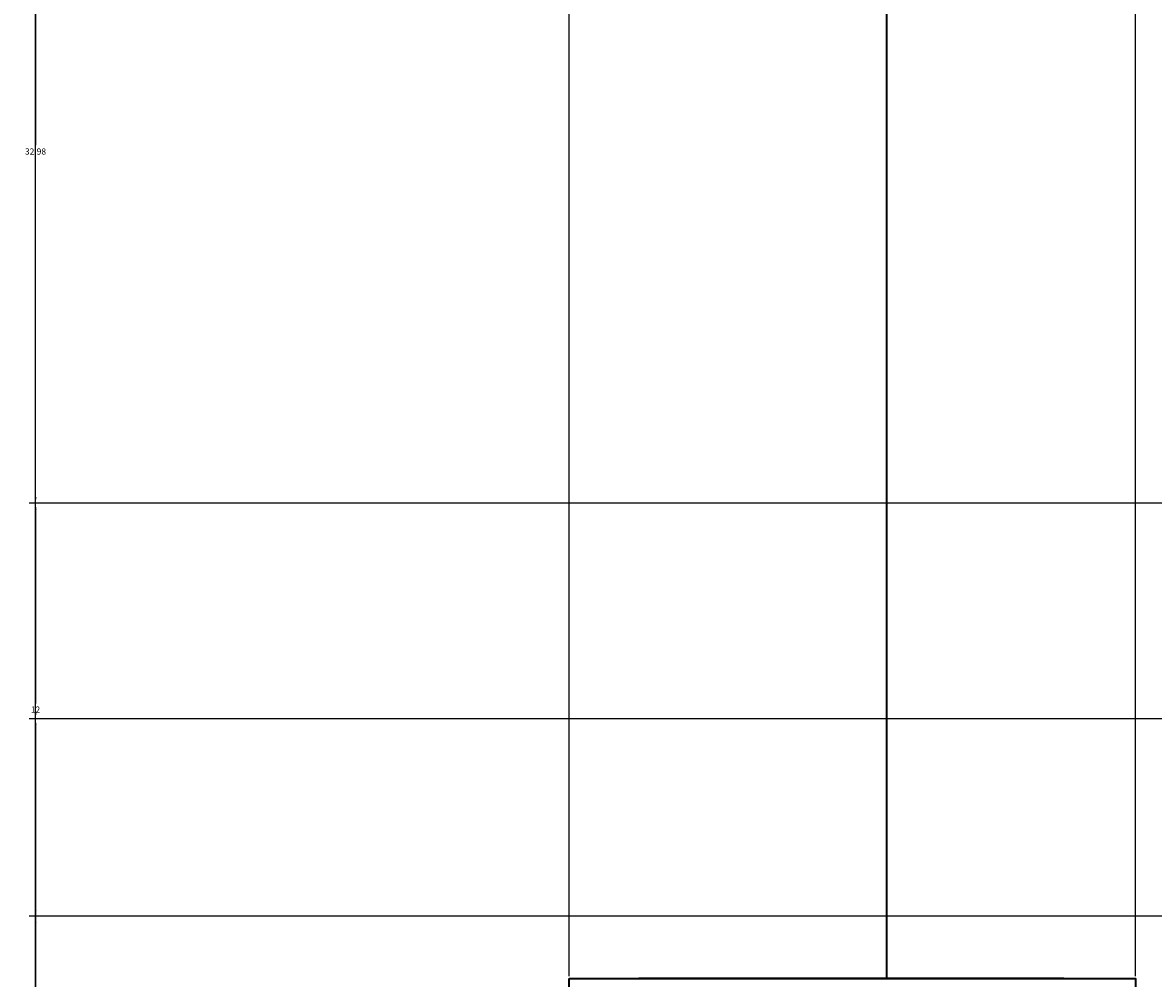
# Model space of a CAD drawing. Units: inches. Extents: x -6 to 289, y -8 to 323.
# Tile 10 of 107: x -6 to 27, y 68 to 96. Entities that reach past the tile are written whole.
import ezdxf

# ---------------------------------------------------------------- set-up
doc = ezdxf.new("R2010")
doc.units = ezdxf.units.IN
doc.header["$MEASUREMENT"] = 0
doc.layers.add('A-ANNO-DIMS', color=2, linetype='Continuous', lineweight=18)
doc.layers.add('A-ELEV', color=7, linetype='Continuous', lineweight=35)
doc.styles.get("Standard").update_dxf_attribs({"font": 'arial.ttf'})
doc.dimstyles.get("Standard").update_dxf_attribs({"dimtxt": 0.18, "dimasz": 0.18, "dimexe": 0.18, "dimexo": 0.0625, "dimgap": 0.09, "dimtad": 0, "dimtih": 1, "dimtoh": 1, "dimdec": 4, "dimzin": 0, "dimdsep": 46, "dimtxsty": 'Standard', "dimcen": 0.09, "dimadec": 0, "dimazin": 0, "dimtfac": 1, "dimtdec": 4, "dimtofl": 0, "dimtmove": 0, "dimatfit": 3, "dimfxl": 1, "dimtolj": 1, "dimtzin": 0, "dimarcsym": 0})

# ---------------------------------------------------------------- blocks, each defined once
blk = doc.blocks.new('*D17')
at = {"layer": 'A-ANNO-DIMS', "color": 0, "lineweight": -2, "transparency": 16777216}
for p, q in [((33.681, 70.243), (-5.737, 70.243)), ((-5.557, 70.063), (-5.557, 38.948)), ((-5.557, 7.469), (-5.557, 38.584)), ((11.907, 7.289), (-5.737, 7.289))]:
    blk.add_line(p, q, dxfattribs=at)
at = {"layer": 'A-ANNO-DIMS', "color": 0, "transparency": 16777216}
for points in [[(-5.587, 70.063), (-5.527, 70.063), (-5.557, 70.243)], [(-5.587, 7.469), (-5.527, 7.469), (-5.557, 7.289)]]:
    blk.add_solid(points, dxfattribs=at)
at = {"layer": 'Defpoints', "color": 0, "transparency": 16777216}
for p in [(-5.557, 70.243), (33.744, 70.243), (11.969, 7.289)]:
    blk.add_point(p, dxfattribs=at)
at = {"layer": 'A-ANNO-DIMS', "color": 0, "transparency": 16777216, "insert": (-5.557, 38.766), "char_height": 0.18, "attachment_point": 5}
blk.add_mtext('\\A1;62.95', dxfattribs=at)
blk = doc.blocks.new('*D18')
at = {"layer": 'A-ANNO-DIMS', "color": 0, "lineweight": -2, "transparency": 16777216}
for p, q in [((45.681, 82.243), (-5.737, 82.243)), ((-5.557, 82.063), (-5.557, 76.423)), ((-5.557, 70.423), (-5.557, 76.062)), ((33.681, 70.243), (-5.737, 70.243))]:
    blk.add_line(p, q, dxfattribs=at)
at = {"layer": 'A-ANNO-DIMS', "color": 0, "transparency": 16777216}
for points in [[(-5.587, 82.063), (-5.527, 82.063), (-5.557, 82.243)], [(-5.587, 70.423), (-5.527, 70.423), (-5.557, 70.243)]]:
    blk.add_solid(points, dxfattribs=at)
at = {"layer": 'Defpoints', "color": 0, "transparency": 16777216}
for p in [(-5.557, 82.243), (45.744, 82.243), (33.744, 70.243)]:
    blk.add_point(p, dxfattribs=at)
at = {"layer": 'A-ANNO-DIMS', "color": 0, "transparency": 16777216, "insert": (-5.557, 76.243), "char_height": 0.18, "attachment_point": 5}
blk.add_mtext('\\A1;12', dxfattribs=at)
blk = doc.blocks.new('*D19')
at = {"layer": 'A-ANNO-DIMS', "color": 0, "lineweight": -2, "transparency": 16777216}
for p, q in [((45.681, 277.043), (-5.737, 277.043)), ((-5.557, 276.863), (-5.557, 179.825)), ((-5.557, 82.423), (-5.557, 179.461)), ((45.681, 82.243), (-5.737, 82.243))]:
    blk.add_line(p, q, dxfattribs=at)
at = {"layer": 'A-ANNO-DIMS', "color": 0, "transparency": 16777216}
for points in [[(-5.587, 276.863), (-5.527, 276.863), (-5.557, 277.043)], [(-5.587, 82.423), (-5.527, 82.423), (-5.557, 82.243)]]:
    blk.add_solid(points, dxfattribs=at)
at = {"layer": 'Defpoints', "color": 0, "transparency": 16777216}
for p in [(-5.557, 277.043), (45.744, 277.043), (45.744, 82.243)]:
    blk.add_point(p, dxfattribs=at)
at = {"layer": 'A-ANNO-DIMS', "color": 0, "transparency": 16777216, "insert": (-5.557, 179.643), "char_height": 0.18, "attachment_point": 5}
blk.add_mtext('\\A1;194.8', dxfattribs=at)
blk = doc.blocks.new('*D22')
at = {"layer": 'A-ANNO-DIMS', "color": 0, "lineweight": -2, "transparency": 16777216}
for p, q in [((19.101, 307.289), (-5.737, 307.289)), ((-5.557, 307.109), (-5.557, 157.471)), ((-5.557, 7.469), (-5.557, 157.107)), ((11.907, 7.289), (-5.737, 7.289))]:
    blk.add_line(p, q, dxfattribs=at)
at = {"layer": 'A-ANNO-DIMS', "color": 0, "transparency": 16777216}
for points in [[(-5.587, 307.109), (-5.527, 307.109), (-5.557, 307.289)], [(-5.587, 7.469), (-5.527, 7.469), (-5.557, 7.289)]]:
    blk.add_solid(points, dxfattribs=at)
at = {"layer": 'Defpoints', "color": 0, "transparency": 16777216}
for p in [(19.164, 307.289), (-5.557, 7.289), (11.969, 7.289)]:
    blk.add_point(p, dxfattribs=at)
at = {"layer": 'A-ANNO-DIMS', "color": 0, "transparency": 16777216, "insert": (-5.557, 157.289), "char_height": 0.18, "attachment_point": 5}
blk.add_mtext('\\A1;300', dxfattribs=at)
blk = doc.blocks.new('*D57')
at = {"layer": 'A-ANNO-DIMS', "color": 0, "lineweight": -2, "transparency": 16777216}
for p, q in [((9.943, 68.495), (9.943, 322.969)), ((26.403, 68.495), (26.403, 322.969)), ((10.123, 322.789), (17.788, 322.789)), ((26.223, 322.789), (18.558, 322.789))]:
    blk.add_line(p, q, dxfattribs=at)
at = {"layer": 'A-ANNO-DIMS', "color": 0, "transparency": 16777216}
for points in [[(10.123, 322.819), (10.123, 322.759), (9.943, 322.789)], [(26.223, 322.819), (26.223, 322.759), (26.403, 322.789)]]:
    blk.add_solid(points, dxfattribs=at)
at = {"layer": 'Defpoints', "color": 0, "transparency": 16777216}
for p in [(26.403, 322.789), (9.943, 68.432), (26.403, 68.432)]:
    blk.add_point(p, dxfattribs=at)
at = {"layer": 'A-ANNO-DIMS', "color": 0, "transparency": 16777216, "insert": (18.173, 322.789), "char_height": 0.18, "attachment_point": 5}
blk.add_mtext('\\A1;16.46', dxfattribs=at)
blk = doc.blocks.new('*D86')
at = {"layer": 'A-ANNO-DIMS', "color": 0, "lineweight": -2, "transparency": 16777216}
for p, q in [((166.233, 75.971), (-5.737, 75.971)), ((-5.557, 75.791), (-5.557, 63.71)), ((-5.557, 51.265), (-5.557, 63.346)), ((120.945, 51.085), (-5.737, 51.085))]:
    blk.add_line(p, q, dxfattribs=at)
at = {"layer": 'A-ANNO-DIMS', "color": 0, "transparency": 16777216}
for points in [[(-5.587, 75.791), (-5.527, 75.791), (-5.557, 75.971)], [(-5.587, 51.265), (-5.527, 51.265), (-5.557, 51.085)]]:
    blk.add_solid(points, dxfattribs=at)
at = {"layer": 'Defpoints', "color": 0, "transparency": 16777216}
for p in [(-5.557, 75.971), (166.296, 75.971), (121.008, 51.085)]:
    blk.add_point(p, dxfattribs=at)
at = {"layer": 'A-ANNO-DIMS', "color": 0, "transparency": 16777216, "insert": (-5.557, 63.528), "char_height": 0.18, "attachment_point": 5}
blk.add_mtext('\\A1;24.886', dxfattribs=at)
blk = doc.blocks.new('*D87')
at = {"layer": 'A-ANNO-DIMS', "color": 0, "lineweight": -2, "transparency": 16777216}
for p, q in [((142.233, 108.948), (-5.737, 108.948)), ((-5.557, 108.768), (-5.557, 92.641)), ((-5.557, 76.151), (-5.557, 92.277)), ((166.233, 75.971), (-5.737, 75.971))]:
    blk.add_line(p, q, dxfattribs=at)
at = {"layer": 'A-ANNO-DIMS', "color": 0, "transparency": 16777216}
for points in [[(-5.587, 108.768), (-5.527, 108.768), (-5.557, 108.948)], [(-5.587, 76.151), (-5.527, 76.151), (-5.557, 75.971)]]:
    blk.add_solid(points, dxfattribs=at)
at = {"layer": 'Defpoints', "color": 0, "transparency": 16777216}
for p in [(-5.557, 108.948), (142.296, 108.948), (166.296, 75.971)]:
    blk.add_point(p, dxfattribs=at)
at = {"layer": 'A-ANNO-DIMS', "color": 0, "transparency": 16777216, "insert": (-5.557, 92.459), "char_height": 0.18, "attachment_point": 5}
blk.add_mtext('\\A1;32.98', dxfattribs=at)

msp = doc.modelspace()

# ---------------------------------------------------------------- linework, layer by layer
at = {"layer": 'A-ELEV'}
msp.add_line((19.1638, 307.2888), (19.1638, 68.4322), dxfattribs=at)
msp.add_lwpolyline([(9.943, 68.4322), (26.403, 68.4322), (26.403, 66.2238), (9.943, 66.2238)], close=True, dxfattribs=at)
msp.add_lwpolyline([(24.317, 68.4322), (11.9692, 68.4322)], dxfattribs=at)

# ---------------------------------------------------------------- dimensions: what is measured, and where the dimension line sits
at = {"layer": 'A-ANNO-DIMS'}
dim = msp.add_linear_dim(base=(26.403, 322.7888), p1=(9.943, 68.4322), p2=(26.403, 68.4322), dimstyle='Standard', override={"dimdec": 2, "dimlfac": 1, "dimrnd": 0, "dimzin": 0, "dimdsep": 46, "dimlunit": 2}, dxfattribs=at)
dim.commit()
dim.dimension.update_dxf_attribs({"geometry": '*D57', "text_midpoint": (18.173, 322.7888)})
for base, p1, p2, override, picture, middle in [((-5.557, 7.2888), (19.1638, 307.2888), (11.9692, 7.2888), {"dimdec": 0, "dimlfac": 1, "dimrnd": 0, "dimzin": 0, "dimdsep": 46, "dimlunit": 2}, '*D22', (-5.557, 157.2888)), ((-5.557, 277.0427), (45.7437, 82.2425), (45.7437, 277.0427), {"dimdec": 1, "dimlfac": 1, "dimrnd": 0, "dimzin": 0, "dimdsep": 46, "dimlunit": 2}, '*D19', (-5.557, 179.6426)), ((-5.557, 108.9477), (166.296, 75.9706), (142.296, 108.9477), {"dimdec": 2, "dimlfac": 1, "dimrnd": 0, "dimzin": 0, "dimdsep": 46, "dimlunit": 2}, '*D87', (-5.557, 92.4592)), ((-5.557, 82.2425), (33.7437, 70.2425), (45.7437, 82.2425), {"dimdec": 0, "dimlfac": 1, "dimrnd": 0, "dimzin": 0, "dimdsep": 46, "dimlunit": 2}, '*D18', (-5.557, 76.2425)), ((-5.557, 75.97064), (121.00798, 51.08513), (166.29599, 75.97064), {"dimdec": 3, "dimlfac": 1, "dimrnd": 0, "dimzin": 0, "dimdsep": 46, "dimlunit": 2}, '*D86', (-5.557, 63.52788)), ((-5.557, 70.2425), (11.9692, 7.2888), (33.7437, 70.2425), {"dimdec": 2, "dimlfac": 1, "dimrnd": 0, "dimzin": 0, "dimdsep": 46, "dimlunit": 2}, '*D17', (-5.557, 38.7657))]:
    dim = msp.add_linear_dim(base=base, p1=p1, p2=p2, angle=90, dimstyle='Standard', override=override, dxfattribs=at)
    dim.commit()
    dim.dimension.update_dxf_attribs({"geometry": picture, "text_midpoint": middle})

doc.saveas('drawing.dxf')
